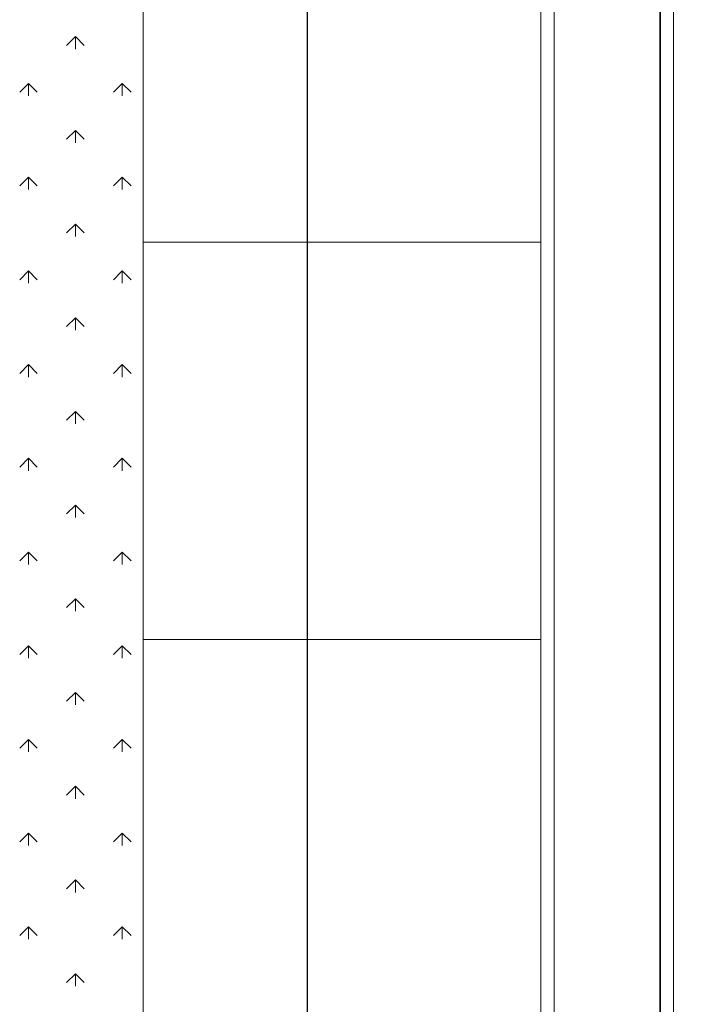
# Model space of a CAD drawing. Units: inches. Extents: x -1198 to -69, y -512 to 437.
# Tile 22 of 50: x -722 to -696, y 39 to 76. Entities that reach past the tile are written whole.
import ezdxf

# ---------------------------------------------------------------- set-up
doc = ezdxf.new("R2010")
doc.units = ezdxf.units.IN
doc.header["$MEASUREMENT"] = 0
for name, color, linetype, lineweight in [('A-ANNO-DIMS', 2, 'Continuous', 18), ('A-FURN', 60, 'Continuous', 18), ('A-WALL', 7, 'Continuous', 35)]:
    doc.layers.add(name, color=color, linetype=linetype, lineweight=lineweight)
doc.styles.get("Standard").update_dxf_attribs({"font": 'arial.ttf'})
doc.dimstyles.get("Standard").update_dxf_attribs({"dimtxt": 6, "dimasz": 6, "dimexe": 0.18, "dimexo": 0.0625, "dimgap": 0.09, "dimtad": 0, "dimtih": 1, "dimtoh": 1, "dimdec": 0, "dimzin": 0, "dimdsep": 46, "dimlunit": 4, "dimtxsty": 'Standard', "dimblk": 'OBLIQUE', "dimcen": 0.09, "dimadec": 0, "dimazin": 0, "dimtfac": 1, "dimtdec": 0, "dimtofl": 0, "dimtmove": 0, "dimatfit": 3, "dimfxl": 1, "dimtolj": 1, "dimtzin": 0, "dimarcsym": 0})

# ---------------------------------------------------------------- blocks, each defined once
blk = doc.blocks.new('A$C3B9F700E')
for p, q in [((736.9, 2080, -685.7), (2936.9, 2080, -685.7)), ((756.9, 2060, -685.7), (2916.9, 2060, -685.7)), ((2916.9, 1900, -685.7), (756.9, 1900, -685.7)), ((2936.9, 1880, -685.7), (736.9, 1880, -685.7)), ((2936.9, 1880, -685.7), (736.9, 1880, -685.7)), ((1536.9, 1880, -685.7), (1536.9, 1280, -685.7)), ((2136.9, 1880, -685.7), (2136.9, 1280, -685.7)), ((2736.9, 1280, -685.7), (936.9, 1280, -685.7)), ((1297.5, 1248.4, -685.7), (1310.8, 1261.7, -685.7)), ((1297.5, 1248.4, -685.7), (1310.8, 1235.2, -685.7)), ((1297.5, 1248.4, -685.7), (1316.3, 1248.4, -685.7)), ((1439, 1248.4, -685.7), (1452.2, 1261.7, -685.7)), ((1439, 1248.4, -685.7), (1452.2, 1235.2, -685.7)), ((1439, 1248.4, -685.7), (1457.7, 1248.4, -685.7)), ((1580.4, 1248.4, -685.7), (1593.6, 1261.7, -685.7)), ((1580.4, 1248.4, -685.7), (1593.6, 1235.2, -685.7)), ((1580.4, 1248.4, -685.7), (1599.1, 1248.4, -685.7)), ((1721.8, 1248.4, -685.7), (1735.1, 1261.7, -685.7)), ((1721.8, 1248.4, -685.7), (1735.1, 1235.2, -685.7)), ((1721.8, 1248.4, -685.7), (1740.6, 1248.4, -685.7)), ((1863.2, 1248.4, -685.7), (1876.5, 1261.7, -685.7)), ((1863.2, 1248.4, -685.7), (1876.5, 1235.2, -685.7)), ((1863.2, 1248.4, -685.7), (1882, 1248.4, -685.7)), ((2004.7, 1248.4, -685.7), (2017.9, 1261.7, -685.7)), ((2004.7, 1248.4, -685.7), (2017.9, 1235.2, -685.7)), ((2004.7, 1248.4, -685.7), (2023.4, 1248.4, -685.7)), ((2146.1, 1248.4, -685.7), (2159.3, 1261.7, -685.7)), ((2146.1, 1248.4, -685.7), (2159.3, 1235.2, -685.7)), ((2146.1, 1248.4, -685.7), (2164.8, 1248.4, -685.7)), ((2287.5, 1248.4, -685.7), (2300.8, 1261.7, -685.7)), ((2287.5, 1248.4, -685.7), (2300.8, 1235.2, -685.7)), ((2287.5, 1248.4, -685.7), (2306.2, 1248.4, -685.7)), ((2428.9, 1248.4, -685.7), (2442.2, 1261.7, -685.7)), ((2428.9, 1248.4, -685.7), (2442.2, 1235.2, -685.7)), ((2428.9, 1248.4, -685.7), (2447.7, 1248.4, -685.7)), ((2570.3, 1248.4, -685.7), (2583.6, 1261.7, -685.7)), ((2570.3, 1248.4, -685.7), (2589.1, 1248.4, -685.7)), ((2570.3, 1248.4, -685.7), (2583.6, 1235.2, -685.7)), ((1226.8, 1177.7, -685.7), (1240.1, 1191, -685.7)), ((1368.3, 1177.7, -685.7), (1381.5, 1191, -685.7)), ((1509.7, 1177.7, -685.7), (1522.9, 1191, -685.7)), ((1651.1, 1177.7, -685.7), (1664.4, 1191, -685.7)), ((1792.5, 1177.7, -685.7), (1805.8, 1191, -685.7)), ((1933.9, 1177.7, -685.7), (1947.2, 1191, -685.7)), ((2075.4, 1177.7, -685.7), (2088.6, 1191, -685.7)), ((2216.8, 1177.7, -685.7), (2230, 1191, -685.7)), ((2358.2, 1177.7, -685.7), (2371.5, 1191, -685.7)), ((2499.6, 1177.7, -685.7), (2512.9, 1191, -685.7)), ((2641.1, 1177.7, -685.7), (2654.3, 1191, -685.7)), ((1226.8, 1177.7, -685.7), (1240.1, 1164.5, -685.7)), ((1226.8, 1177.7, -685.7), (1245.6, 1177.7, -685.7)), ((1368.3, 1177.7, -685.7), (1381.5, 1164.5, -685.7)), ((1368.3, 1177.7, -685.7), (1387, 1177.7, -685.7)), ((1509.7, 1177.7, -685.7), (1522.9, 1164.5, -685.7)), ((1509.7, 1177.7, -685.7), (1528.4, 1177.7, -685.7)), ((1651.1, 1177.7, -685.7), (1664.4, 1164.5, -685.7)), ((1651.1, 1177.7, -685.7), (1669.9, 1177.7, -685.7)), ((1792.5, 1177.7, -685.7), (1805.8, 1164.5, -685.7)), ((1792.5, 1177.7, -685.7), (1811.3, 1177.7, -685.7)), ((1933.9, 1177.7, -685.7), (1947.2, 1164.5, -685.7)), ((1933.9, 1177.7, -685.7), (1952.7, 1177.7, -685.7)), ((2075.4, 1177.7, -685.7), (2088.6, 1164.5, -685.7)), ((2075.4, 1177.7, -685.7), (2094.1, 1177.7, -685.7)), ((2216.8, 1177.7, -685.7), (2230, 1164.5, -685.7)), ((2216.8, 1177.7, -685.7), (2235.5, 1177.7, -685.7)), ((2358.2, 1177.7, -685.7), (2371.5, 1164.5, -685.7)), ((2358.2, 1177.7, -685.7), (2377, 1177.7, -685.7)), ((2499.6, 1177.7, -685.7), (2512.9, 1164.5, -685.7)), ((2499.6, 1177.7, -685.7), (2518.4, 1177.7, -685.7)), ((2641.1, 1177.7, -685.7), (2654.3, 1164.5, -685.7)), ((2641.1, 1177.7, -685.7), (2659.8, 1177.7, -685.7)), ((1297.5, 1107, -685.7), (1310.8, 1120.3, -685.7)), ((1439, 1107, -685.7), (1452.2, 1120.3, -685.7)), ((1580.4, 1107, -685.7), (1593.6, 1120.3, -685.7)), ((1721.8, 1107, -685.7), (1735.1, 1120.3, -685.7)), ((1863.2, 1107, -685.7), (1876.5, 1120.3, -685.7)), ((2004.7, 1107, -685.7), (2017.9, 1120.3, -685.7)), ((2146.1, 1107, -685.7), (2159.3, 1120.3, -685.7)), ((2287.5, 1107, -685.7), (2300.8, 1120.3, -685.7)), ((2428.9, 1107, -685.7), (2442.2, 1120.3, -685.7)), ((2570.3, 1107, -685.7), (2583.6, 1120.3, -685.7)), ((1297.5, 1107, -685.7), (1310.8, 1093.8, -685.7)), ((1297.5, 1107, -685.7), (1316.3, 1107, -685.7)), ((1439, 1107, -685.7), (1452.2, 1093.8, -685.7)), ((1439, 1107, -685.7), (1457.7, 1107, -685.7)), ((1580.4, 1107, -685.7), (1593.6, 1093.8, -685.7)), ((1580.4, 1107, -685.7), (1599.1, 1107, -685.7)), ((1721.8, 1107, -685.7), (1735.1, 1093.8, -685.7)), ((1721.8, 1107, -685.7), (1740.6, 1107, -685.7)), ((1863.2, 1107, -685.7), (1876.5, 1093.8, -685.7)), ((1863.2, 1107, -685.7), (1882, 1107, -685.7)), ((2004.7, 1107, -685.7), (2017.9, 1093.8, -685.7)), ((2004.7, 1107, -685.7), (2023.4, 1107, -685.7)), ((2146.1, 1107, -685.7), (2159.3, 1093.8, -685.7)), ((2146.1, 1107, -685.7), (2164.8, 1107, -685.7)), ((2287.5, 1107, -685.7), (2300.8, 1093.8, -685.7)), ((2287.5, 1107, -685.7), (2306.2, 1107, -685.7)), ((2428.9, 1107, -685.7), (2442.2, 1093.8, -685.7)), ((2428.9, 1107, -685.7), (2447.7, 1107, -685.7)), ((2570.3, 1107, -685.7), (2589.1, 1107, -685.7)), ((2570.3, 1107, -685.7), (2583.6, 1093.8, -685.7))]:
    blk.add_line(p, q)
blk = doc.blocks.new('1')
blk.add_blockref('A$C3B9F700E', (-1861.1, 172.7, 685.7))
blk = doc.blocks.new('_Oblique')
at = {"color": 0, "linetype": 'ByBlock', "lineweight": -2}
blk.add_line((-0.5, -0.5), (0.5, 0.5), dxfattribs=at)
blk = doc.blocks.new('*D76')
at = {"layer": 'A-ANNO-DIMS', "color": 0, "lineweight": -2, "ltscale": 10, "transparency": 16777216}
for p, q in [((-711.132, -38.21), (-711.132, 433.184)), ((-697.751, -38.21), (-697.751, 433.184)), ((-711.132, 433.004), (-697.751, 433.004)), ((-697.751, 433.004), (-691.751, 433.004))]:
    blk.add_line(p, q, dxfattribs=at)
at = {"layer": 'DEFPOINTS', "color": 0, "ltscale": 10, "transparency": 16777216}
for p in [(-697.751, 433.004), (-711.132, -38.272), (-697.751, -38.272)]:
    blk.add_point(p, dxfattribs=at)
at = {"layer": 'A-ANNO-DIMS', "color": 0, "lineweight": -2, "ltscale": 10, "transparency": 16777216, "xscale": 6, "yscale": 6, "zscale": 6, "rotation": 180}
blk.add_blockref('_Oblique', (-711.132, 433.004), dxfattribs=at)
at = {"layer": 'A-ANNO-DIMS', "color": 0, "lineweight": -2, "ltscale": 10, "transparency": 16777216, "xscale": 6, "yscale": 6, "zscale": 6}
blk.add_blockref('_Oblique', (-697.751, 433.004), dxfattribs=at)
at = {"layer": 'A-ANNO-DIMS', "color": 0, "ltscale": 10, "transparency": 16777216, "insert": (-681.814, 433.004), "char_height": 6, "attachment_point": 5}
blk.add_mtext('\\A1;13.38', dxfattribs=at)

msp = doc.modelspace()

# ---------------------------------------------------------------- linework, layer by layer
at = {"layer": 'A-WALL', "ltscale": 10}
msp.add_line((-697.7509, 158.2277), (-697.7509, 35.2277), dxfattribs=at)

# ---------------------------------------------------------------- block references
at = {"layer": 'A-FURN', "ltscale": 10, "xscale": 0.0251614738227896, "yscale": 0.0251614738227896, "zscale": 0.0251614738227896, "rotation": 270.0000000000001}
msp.add_blockref('1', (-753.9284, 59.7223), dxfattribs=at)

# ---------------------------------------------------------------- dimensions: what is measured, and where the dimension line sits
at = {"layer": 'A-ANNO-DIMS', "ltscale": 10}
dim = msp.add_linear_dim(base=(-697.7509, 433.0036), p1=(-711.1319, -38.2723), p2=(-697.7509, -38.2723), dimstyle='Standard', override={"dimdec": 2, "dimlfac": 1, "dimrnd": 0, "dimzin": 0, "dimdsep": 46, "dimlunit": 2}, dxfattribs=at)
dim.commit()
dim.dimension.update_dxf_attribs({"geometry": '*D76', "text_midpoint": (-681.8137, 433.0036)})

doc.saveas('drawing.dxf')
